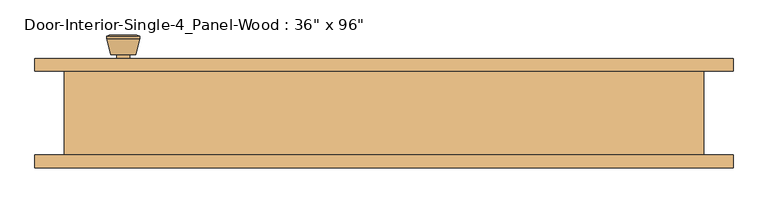
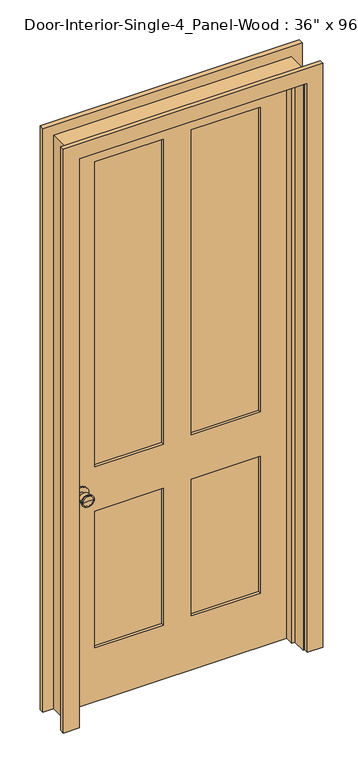
"""IFC4 building model written with IfcOpenShell, lengths in millimetres: door geometry."""

from ifc_helpers import new_model, si_unit, point, frame, frame_2d, origin, place, context, project, spatial, polyline, circle_curve, trimmed, segment, composite_curve, outline, extrude, faceted_brep, source, transform, mapped, element, save
from ifc_brep_helpers import plane_surface, cylinder_surface, revolved_surface, advanced_brep


def door_72f69035(model_context):
    return source(origin(), model_context, "Body", "SolidModel", [
        advanced_brep(
        [(-393.7, 19.4, 914.4), (-383.7, 19.4, 914.4), (-403.7, 19.4, 914.4), (-373.2241324, -29.6, 914.4), (-393.7, -29.6, 914.4), (-414.1758676, -29.6, 914.4), (-368.7, -27.7721319, 914.4), (-418.7, -27.7721319, 914.4), (-368.7, -24.3084537, 914.4), (-418.7, -24.3084537, 914.4), (-375.063764, 0.4, 914.4), (-412.336236, 0.4, 914.4), (-383.7, 0.4, 914.4), (-403.7, 0.4, 914.4)],
        [
            (0, 1),
            (1, 2, circle_curve(frame((-393.7, 19.4, 914.4), z_axis=(0.0, 1.0, 0.0), x_axis=(-1.0, 0.0, 0.0)), 10.0)),
            (2, 0),
            (2, 1, circle_curve(frame((-393.7, 19.4, 914.4), z_axis=(0.0, 1.0, 0.0), x_axis=(-1.0, 0.0, 0.0)), 10.0)),
            (3, 4),
            (4, 5),
            (5, 3, circle_curve(frame((-393.7, -29.6, 914.4), z_axis=(0.0, -1.0, 0.0), x_axis=(-1.0, 0.0, 0.0)), 20.4758676)),
            (3, 5, circle_curve(frame((-393.7, -29.6, 914.4), z_axis=(0.0, -1.0, 0.0), x_axis=(-1.0, 0.0, 0.0)), 20.4758676)),
            (6, 3),
            (5, 7),
            (7, 6, circle_curve(frame((-393.7, -27.7721319, 914.4), z_axis=(0.0, -1.0, 0.0), x_axis=(-1.0, 0.0, 0.0)), 25.0)),
            (6, 7, circle_curve(frame((-393.7, -27.7721319, 914.4), z_axis=(0.0, -1.0, 0.0), x_axis=(-1.0, 0.0, 0.0)), 25.0)),
            (8, 6),
            (7, 9),
            (9, 8, circle_curve(frame((-393.7, -24.3084537, 914.4), z_axis=(0.0, -1.0, 0.0), x_axis=(-1.0, 0.0, 0.0)), 25.0)),
            (8, 9, circle_curve(frame((-393.7, -24.3084537, 914.4), z_axis=(0.0, -1.0, 0.0), x_axis=(-1.0, 0.0, 0.0)), 25.0)),
            (10, 8),
            (9, 11),
            (11, 10, circle_curve(frame((-393.7, 0.4, 914.4), z_axis=(0.0, -1.0, 0.0), x_axis=(-1.0, 0.0, 0.0)), 18.636236)),
            (10, 11, circle_curve(frame((-393.7, 0.4, 914.4), z_axis=(0.0, -1.0, 0.0), x_axis=(-1.0, 0.0, 0.0)), 18.636236)),
            (12, 10),
            (11, 13),
            (13, 12, circle_curve(frame((-393.7, 0.4, 914.4), z_axis=(0.0, -1.0, 0.0), x_axis=(-1.0, 0.0, 0.0)), 10.0)),
            (12, 13, circle_curve(frame((-393.7, 0.4, 914.4), z_axis=(0.0, -1.0, 0.0), x_axis=(-1.0, 0.0, 0.0)), 10.0)),
            (1, 12),
            (13, 2),
        ],
        [
            plane_surface(frame((-393.7, 19.4, 914.4), z_axis=(0.0, 1.0, 0.0), x_axis=(-1.0, 0.0, 0.0))),
            plane_surface(frame((-393.7, -29.6, 914.4), z_axis=(0.0, -1.0, 0.0), x_axis=(-1.0, 0.0, 0.0))),
            revolved_surface(polyline([(-414.1758676, -29.6, 914.4), (-418.7, -27.7721319, 914.4)]), (-393.7, 19.4, 914.4), (0.0, 1.0, 0.0)),
            cylinder_surface(frame((-393.7, 19.4, 914.4), z_axis=(0.0, 1.0, 0.0), x_axis=(-1.0, 0.0, 0.0)), 25.0),
            revolved_surface(polyline([(-418.7, -24.3084537, 914.4), (-412.336236, 0.4, 914.4)]), (-393.7, 19.4, 914.4), (0.0, 1.0, 0.0)),
            plane_surface(frame((-393.7, 0.4, 914.4), z_axis=(0.0, 1.0, 0.0), x_axis=(-1.0, 0.0, 0.0))),
            cylinder_surface(frame((-393.7, 19.4, 914.4), z_axis=(0.0, 1.0, 0.0), x_axis=(-1.0, 0.0, 0.0)), 10.0),
        ],
        [
            (0, [[1, 2, 3]]),
            (0, [[-3, 4, -1]]),
            (1, [[5, 6, 7]]),
            (1, [[-6, -5, 8]]),
            (2, [[9, -7, 10, 11]]),
            (2, [[-10, -8, -9, 12]]),
            (3, [[13, -11, 14, 15]]),
            (3, [[-14, -12, -13, 16]]),
            (4, [[17, -15, 18, 19]]),
            (4, [[-18, -16, -17, 20]]),
            (5, [[21, -19, 22, 23]]),
            (5, [[-22, -20, -21, 24]]),
            (6, [[25, -23, 26, -2]]),
            (6, [[-26, -24, -25, -4]]),
        ],
    ),
        extrude(outline(composite_curve([segment(trimmed(circle_curve(frame_2d((914.4, -393.7)), 30.0), [point((914.4, -423.7))], [point((914.4, -363.7))], False, "CARTESIAN"), True, "CONTINUOUS"), segment(trimmed(circle_curve(frame_2d((914.4, -393.7)), 30.0), [point((914.4, -363.7))], [point((914.4, -423.7))], False, "CARTESIAN"), True, "CONTINUOUS")], self_intersect=False)), frame((0.0, 19.4, 0.0), z_axis=(0.0, 1.0, 0.0), x_axis=(0.0, 0.0, 1.0)), (0.0, 0.0, 1.0), 6.0),
        advanced_brep(
        [(-393.7, 66.325, 914.4), (-403.7, 66.325, 914.4), (-383.7, 66.325, 914.4), (-373.2241324, 115.325, 914.4), (-414.1758676, 115.325, 914.4), (-393.7, 115.325, 914.4), (-368.7, 113.4971319, 914.4), (-418.7, 113.4971319, 914.4), (-368.7, 110.0334537, 914.4), (-418.7, 110.0334537, 914.4), (-375.063764, 85.325, 914.4), (-412.336236, 85.325, 914.4), (-383.7, 85.325, 914.4), (-403.7, 85.325, 914.4)],
        [
            (0, 1),
            (1, 2, circle_curve(frame((-393.7, 66.325, 914.4), z_axis=(0.0, -1.0, 0.0), x_axis=(-1.0, 0.0, 0.0)), 10.0)),
            (2, 0),
            (2, 1, circle_curve(frame((-393.7, 66.325, 914.4), z_axis=(0.0, -1.0, 0.0), x_axis=(-1.0, 0.0, 0.0)), 10.0)),
            (3, 4, circle_curve(frame((-393.7, 115.325, 914.4), z_axis=(0.0, 1.0, 0.0), x_axis=(-1.0, 0.0, 0.0)), 20.4758676)),
            (4, 5),
            (5, 3),
            (4, 3, circle_curve(frame((-393.7, 115.325, 914.4), z_axis=(0.0, 1.0, 0.0), x_axis=(-1.0, 0.0, 0.0)), 20.4758676)),
            (6, 7, circle_curve(frame((-393.7, 113.4971319, 914.4), z_axis=(0.0, 1.0, 0.0), x_axis=(-1.0, 0.0, 0.0)), 25.0)),
            (7, 4),
            (3, 6),
            (7, 6, circle_curve(frame((-393.7, 113.4971319, 914.4), z_axis=(0.0, 1.0, 0.0), x_axis=(-1.0, 0.0, 0.0)), 25.0)),
            (8, 9, circle_curve(frame((-393.7, 110.0334537, 914.4), z_axis=(0.0, 1.0, 0.0), x_axis=(-1.0, 0.0, 0.0)), 25.0)),
            (9, 7),
            (6, 8),
            (9, 8, circle_curve(frame((-393.7, 110.0334537, 914.4), z_axis=(0.0, 1.0, 0.0), x_axis=(-1.0, 0.0, 0.0)), 25.0)),
            (10, 11, circle_curve(frame((-393.7, 85.325, 914.4), z_axis=(0.0, 1.0, 0.0), x_axis=(-1.0, 0.0, 0.0)), 18.636236)),
            (11, 9),
            (8, 10),
            (11, 10, circle_curve(frame((-393.7, 85.325, 914.4), z_axis=(0.0, 1.0, 0.0), x_axis=(-1.0, 0.0, 0.0)), 18.636236)),
            (12, 13, circle_curve(frame((-393.7, 85.325, 914.4), z_axis=(0.0, 1.0, 0.0), x_axis=(-1.0, 0.0, 0.0)), 10.0)),
            (13, 11),
            (10, 12),
            (13, 12, circle_curve(frame((-393.7, 85.325, 914.4), z_axis=(0.0, 1.0, 0.0), x_axis=(-1.0, 0.0, 0.0)), 10.0)),
            (1, 13),
            (12, 2),
        ],
        [
            plane_surface(frame((-393.7, 66.325, 914.4), z_axis=(0.0, -1.0, 0.0), x_axis=(-1.0, 0.0, 0.0))),
            plane_surface(frame((-393.7, 115.325, 914.4), z_axis=(0.0, 1.0, 0.0), x_axis=(-1.0, 0.0, 0.0))),
            revolved_surface(polyline([(-414.1758676, 115.325, 914.4), (-418.7, 113.4971319, 914.4)]), (-393.7, 66.325, 914.4), (0.0, -1.0, 0.0)),
            cylinder_surface(frame((-393.7, 66.325, 914.4), z_axis=(0.0, -1.0, 0.0), x_axis=(-1.0, 0.0, 0.0)), 25.0),
            revolved_surface(polyline([(-418.7, 110.0334537, 914.4), (-412.336236, 85.325, 914.4)]), (-393.7, 66.325, 914.4), (0.0, -1.0, 0.0)),
            plane_surface(frame((-393.7, 85.325, 914.4), z_axis=(0.0, -1.0, 0.0), x_axis=(-1.0, 0.0, 0.0))),
            cylinder_surface(frame((-393.7, 66.325, 914.4), z_axis=(0.0, -1.0, 0.0), x_axis=(-1.0, 0.0, 0.0)), 10.0),
        ],
        [
            (0, [[1, 2, 3]]),
            (0, [[-3, 4, -1]]),
            (1, [[5, 6, 7]]),
            (1, [[8, -7, -6]]),
            (2, [[9, 10, -5, 11]]),
            (2, [[12, -11, -8, -10]]),
            (3, [[13, 14, -9, 15]]),
            (3, [[16, -15, -12, -14]]),
            (4, [[17, 18, -13, 19]]),
            (4, [[20, -19, -16, -18]]),
            (5, [[21, 22, -17, 23]]),
            (5, [[24, -23, -20, -22]]),
            (6, [[-2, 25, -21, 26]]),
            (6, [[-4, -26, -24, -25]]),
        ],
    ),
        extrude(outline(composite_curve([segment(trimmed(circle_curve(frame_2d((914.4, -393.7)), 30.0), [point((914.4, -423.7))], [point((914.4, -363.7))], False, "CARTESIAN"), True, "CONTINUOUS"), segment(trimmed(circle_curve(frame_2d((914.4, -393.7)), 30.0), [point((914.4, -363.7))], [point((914.4, -423.7))], False, "CARTESIAN"), True, "CONTINUOUS")], self_intersect=False)), frame((0.0, 60.325, 0.0), z_axis=(0.0, 1.0, 0.0), x_axis=(0.0, 0.0, 1.0)), (0.0, 0.0, 1.0), 6.0),
        faceted_brep([(482.6, 60.325, 0.0), (482.6, -66.675, 0.0), (457.2, -66.675, 0.0), (457.2, -9.525, 0.0), (444.5, -9.525, 0.0), (444.5, 25.4, 0.0), (457.2, 25.4, 0.0), (457.2, 60.325, 0.0), (482.6, 60.325, 2463.8), (482.6, -66.675, 2463.8), (-482.6, -66.675, 2463.8), (-482.6, -66.675, 0.0), (-457.2, -66.675, 0.0), (-457.2, -66.675, 2438.4), (457.2, -66.675, 2438.4), (457.2, -9.525, 2438.4), (-457.2, -9.525, 2438.4), (-457.2, -9.525, 0.0), (-444.5, -9.525, 0.0), (-444.5, -9.525, 2425.7), (444.5, -9.525, 2425.7), (444.5, 25.4, 2425.7), (-444.5, 25.4, 2425.7), (-444.5, 25.4, 0.0), (-457.2, 25.4, 0.0), (-457.2, 25.4, 2438.4), (457.2, 25.4, 2438.4), (457.2, 60.325, 2438.4), (-457.2, 60.325, 2438.4), (-457.2, 60.325, 0.0), (-482.6, 60.325, 0.0), (-482.6, 60.325, 2463.8)], [[[0, 1, 2, 3, 4, 5, 6, 7]], [[1, 0, 8, 9]], [[2, 1, 9, 10, 11, 12, 13, 14]], [[3, 2, 14, 15]], [[4, 3, 15, 16, 17, 18, 19, 20]], [[5, 4, 20, 21]], [[6, 5, 21, 22, 23, 24, 25, 26]], [[7, 6, 26, 27]], [[0, 7, 27, 28, 29, 30, 31, 8]], [[9, 8, 31, 10]], [[15, 14, 13, 16]], [[21, 20, 19, 22]], [[27, 26, 25, 28]], [[30, 29, 24, 23, 18, 17, 12, 11]], [[10, 31, 30, 11]], [[16, 13, 12, 17]], [[22, 19, 18, 23]], [[28, 25, 24, 29]]]),
        extrude(outline(polyline([(2438.4, -457.2), (0.0, -457.2), (0.0, 457.2), (2438.4, 457.2), (2438.4, -457.2)]), holes=[polyline([(2319.3375, 57.15), (2319.3375, 336.55), (1009.65, 336.55), (1009.65, 57.15), (2319.3375, 57.15)]), polyline([(1009.65, -57.15), (1009.65, -336.55), (2319.3375, -336.55), (2319.3375, -57.15), (1009.65, -57.15)]), polyline([(819.15, 57.15), (819.15, 336.55), (231.775, 336.55), (231.775, 57.15), (819.15, 57.15)]), polyline([(231.775, -57.15), (231.775, -336.55), (819.15, -336.55), (819.15, -57.15), (231.775, -57.15)])]), frame((0.0, 25.4, 0.0), z_axis=(0.0, 1.0, 0.0), x_axis=(0.0, 0.0, 1.0)), (0.0, 0.0, 1.0), 34.925),
        extrude(outline(polyline([(336.55, 37.0416667), (57.15, 37.0416667), (57.15, 48.6833333), (336.55, 48.6833333), (336.55, 37.0416667)])), frame((0.0, 0.0, 1009.65), z_axis=(0.0, 0.0, 1.0), x_axis=(1.0, 0.0, 0.0)), (0.0, 0.0, 1.0), 1309.6875),
        extrude(outline(polyline([(-57.15, 37.0416667), (-336.55, 37.0416667), (-336.55, 48.6833333), (-57.15, 48.6833333), (-57.15, 37.0416667)])), frame((0.0, 0.0, 1009.65), z_axis=(0.0, 0.0, 1.0), x_axis=(1.0, 0.0, 0.0)), (0.0, 0.0, 1.0), 1309.6875),
        extrude(outline(polyline([(336.55, 37.0416667), (57.15, 37.0416667), (57.15, 48.6833333), (336.55, 48.6833333), (336.55, 37.0416667)])), frame((0.0, 0.0, 231.775), z_axis=(0.0, 0.0, 1.0), x_axis=(1.0, 0.0, 0.0)), (0.0, 0.0, 1.0), 587.375),
        extrude(outline(polyline([(-57.15, 37.0416667), (-336.55, 37.0416667), (-336.55, 48.6833333), (-57.15, 48.6833333), (-57.15, 37.0416667)])), frame((0.0, 0.0, 231.775), z_axis=(0.0, 0.0, 1.0), x_axis=(1.0, 0.0, 0.0)), (0.0, 0.0, 1.0), 587.375),
        extrude(outline(polyline([(0.0, 463.55), (0.0, 527.05), (2508.25, 527.05), (2508.25, -527.05), (0.0, -527.05), (0.0, -463.55), (2444.75, -463.55), (2444.75, 463.55), (0.0, 463.55)])), frame((0.0, 60.325, 0.0), z_axis=(0.0, 1.0, 0.0), x_axis=(0.0, 0.0, 1.0)), (0.0, 0.0, 1.0), 19.05),
        extrude(outline(polyline([(0.0, 463.55), (0.0, 527.05), (2508.25, 527.05), (2508.25, -527.05), (0.0, -527.05), (0.0, -463.55), (2444.75, -463.55), (2444.75, 463.55), (0.0, 463.55)])), frame((0.0, -85.725, 0.0), z_axis=(0.0, 1.0, 0.0), x_axis=(0.0, 0.0, 1.0)), (0.0, 0.0, 1.0), 19.05),
    ])


if __name__ == "__main__":
    model = new_model("IFC4")
    model_context = context("Model", 3, world=origin())
    ifc_project = project(units=[si_unit("LENGTHUNIT", "METRE", prefix="MILLI")], contexts=[model_context])
    site = spatial("IfcSite", under=ifc_project)
    building = spatial("IfcBuilding", under=site)
    placement = place(None, origin())
    door_shape = door_72f69035(model_context)
    element("IfcDoor", 1, ObjectType="Door-Interior-Single-4_Panel-Wood : 36\" x 96\"", at=placement, inside=building, context=model_context, shape_type="MappedRepresentation", body=[
        mapped(door_shape, transform((0.0, 0.0, 0.0), x_axis=(1.0, 0.0, 0.0), y_axis=(0.0, 1.0, 0.0), z_axis=(0.0, 0.0, 1.0))),
    ])
    save(model, "model.ifc")

# Revit data of these elements
# Type "Door-Interior-Single-4_Panel-Wood : 36\" x 96\""
#   Type Mark = "9"
#   Assembly Code = "C1020300"
#   Analytic Construction = "Wooden"
#   Top Rail = 0' - 4 11/16"
#   Thickness = 0' - 1 3/8"
#   Thermal Resistance (R) = 2.5876 (h·ft²·°F)/BTU
#   Swing Angle [instance default] = 90.00°
#   Stiles = 0' - 4 3/4"
#   Rough Width = 3' - 2"
#   Rough Height = 8' - 1"
#   Mullion = 0' - 4 1/2"
#   Lock Rail = 0' - 7 1/2"
#   Height = 8' - 0"
#   Width = 3' - 0"
#   Heat Transfer Coefficient (U) = 0.3865 BTU/(h·ft²·°F)
#   Bottom Rail = 0' - 9 1/8"
#   Trim Material = Cherry
#   Panel Material = Cherry
#   Frame Material = Cherry
#   Door Handle Material = Aluminum
#   Visual Light Transmittance = 0
#   Solar Heat Gain Coefficient = 0
#   Wall Closure = (empty or 0)
#   Function = (empty or 0)
# Element 1 (IfcDoor, "Door-Interior-Single-4_Panel-Wood : 36\" x 96\"")
#   Materials on its faces: "Cherry", "Aluminum"
# Materials
#   "Cherry": class "Wood", colour RGB 226 177 128, transparency 0, Description = "Prunus Serotina", Cost = 0
#   "Aluminum": class "Metal", colour RGB 247 247 247, transparency 0, Description = "Aluminum 6061", Cost = 0
